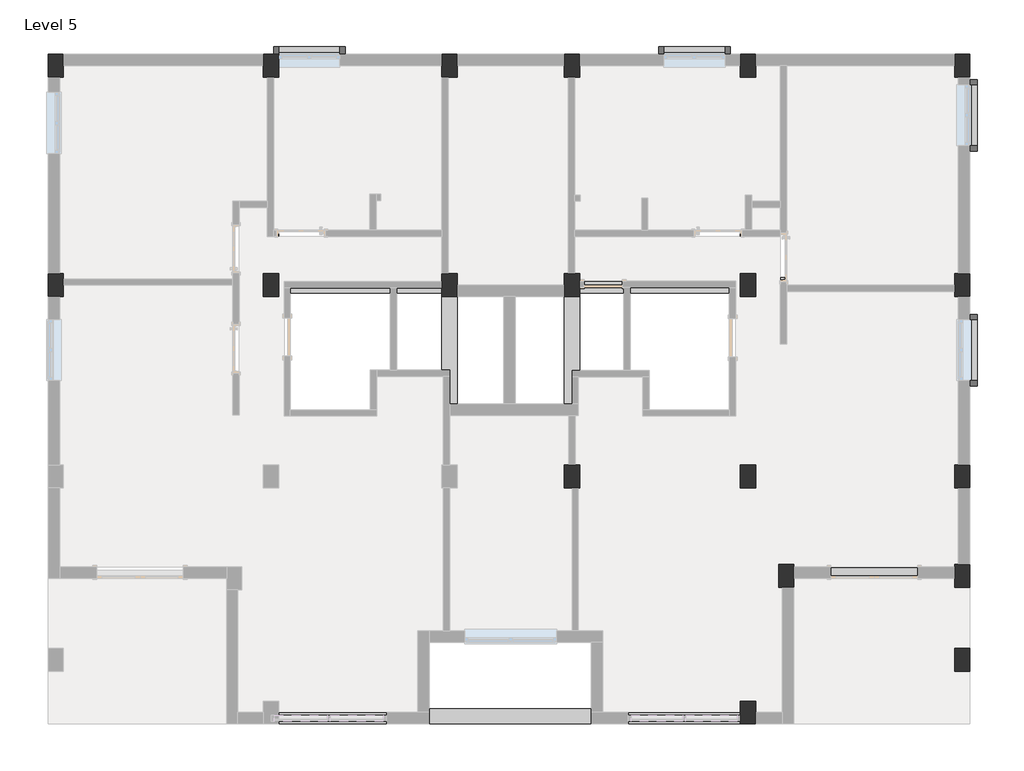
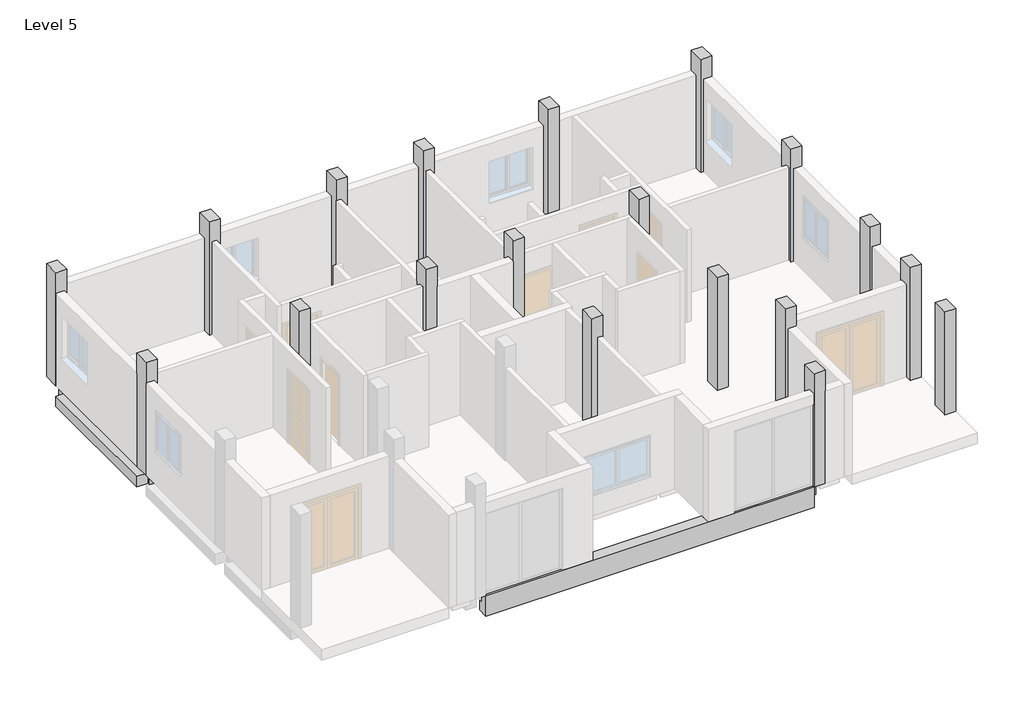
# One storey, part 3 of 3: 30 beams, 19 columns, 4 proxies.
"""IFC4 building model written with IfcOpenShell, lengths in millimetres."""

from ifc_helpers import new_model, si_unit, frame, origin, place, context, project, spatial, polyline, outline, extrude, faceted_brep, transform, mapped, element, save
from components import generic_models_10_generic_models_5_40bb8100, generic_models_13_generic_models_13_6edbfaa0, column_61ecc76d

model = new_model("IFC4")

# Units and contexts
model_context = context("Model", 3, world=origin())
ifc_project = project(units=[si_unit("LENGTHUNIT", "METRE", prefix="MILLI")], contexts=[model_context])

# Site, building, storey
site = spatial("IfcSite", under=ifc_project)
building = spatial("IfcBuilding", under=site)
storey = spatial("IfcBuildingStorey", under=building, Name="Level 5", Elevation=6400.8)

# Beams
placement = place(None, origin())
element("IfcBeam", 1, ObjectType="Concrete-Rectangular Beam : 12 x 24", at=placement, inside=storey, context=model_context, shape_type="SweptSolid", body=[
    extrude(outline(polyline([(-8839.9786397, -1604.6061634), (-8839.9786397, -1299.8061634), (-4852.9175798, -1299.8061634), (-4852.9175798, -1604.6061634), (-8839.9786397, -1604.6061634)])), frame((0.0, 0.0, 5791.2), z_axis=(0.0, 0.0, 1.0), x_axis=(1.0, 0.0, 0.0)), (0.0, 0.0, 1.0), 304.8),
])
element("IfcBeam", 2, ObjectType="Concrete-Rectangular Beam : 12 x 24", at=placement, inside=storey, context=model_context, shape_type="SweptSolid", body=[
    extrude(outline(polyline([(-1296.9175798, -1604.6061634), (-4548.1175798, -1604.6061634), (-4548.1175798, -1299.8061634), (-1296.9175798, -1299.8061634), (-1296.9175798, -1604.6061634)])), frame((0.0, 0.0, 5791.2), z_axis=(0.0, 0.0, 1.0), x_axis=(1.0, 0.0, 0.0)), (0.0, 0.0, 1.0), 304.8),
])
element("IfcBeam", 3, ObjectType="Concrete-Rectangular Beam : 12 x 24", at=placement, inside=storey, context=model_context, shape_type="SweptSolid", body=[
    extrude(outline(polyline([(1141.4824202, -1604.6061634), (-992.1175798, -1604.6061634), (-992.1175798, -1299.8061634), (1141.4824202, -1299.8061634), (1141.4824202, -1604.6061634)])), frame((0.0, 0.0, 5791.2), z_axis=(0.0, 0.0, 1.0), x_axis=(1.0, 0.0, 0.0)), (0.0, 0.0, 1.0), 304.8),
])
element("IfcBeam", 4, ObjectType="Concrete-Rectangular Beam : 12 x 24", at=placement, inside=storey, context=model_context, shape_type="SweptSolid", body=[
    extrude(outline(polyline([(4646.6824202, -1604.6061634), (1446.2824202, -1604.6061634), (1446.2824202, -1299.8061634), (4646.6824202, -1299.8061634), (4646.6824202, -1604.6061634)])), frame((0.0, 0.0, 5791.2), z_axis=(0.0, 0.0, 1.0), x_axis=(1.0, 0.0, 0.0)), (0.0, 0.0, 1.0), 304.8),
])
element("IfcBeam", 5, ObjectType="Concrete-Rectangular Beam : 12 x 24", at=placement, inside=storey, context=model_context, shape_type="SweptSolid", body=[
    extrude(outline(polyline([(8913.9345022, -1604.6061634), (4951.5345022, -1604.6061634), (4951.5345022, -1299.8061634), (8913.9345022, -1299.8061634), (8913.9345022, -1604.6061634)])), frame((0.0, 0.0, 5791.2), z_axis=(0.0, 0.0, 1.0), x_axis=(1.0, 0.0, 0.0)), (0.0, 0.0, 1.0), 304.8),
])
element("IfcBeam", 6, ObjectType="Concrete-Rectangular Beam : 12 x 24", at=placement, inside=storey, context=model_context, shape_type="SweptSolid", body=[
    extrude(outline(polyline([(8913.8824202, -5600.6620333), (8913.8824202, -1680.8061634), (9218.6824202, -1680.8061634), (9218.6824202, -5600.6620333), (8913.8824202, -5600.6620333)])), frame((0.0, 0.0, 5791.2), z_axis=(0.0, 0.0, 1.0), x_axis=(1.0, 0.0, 0.0)), (0.0, 0.0, 1.0), 304.8),
])
element("IfcBeam", 7, ObjectType="Concrete-Rectangular Beam : 12 x 24", at=placement, inside=storey, context=model_context, shape_type="SweptSolid", body=[
    extrude(outline(polyline([(8913.8824202, -9410.6620333), (8913.8824202, -6057.8620333), (9218.6824202, -6057.8620333), (9218.6824202, -9410.6620333), (8913.8824202, -9410.6620333)])), frame((0.0, 0.0, 5791.2), z_axis=(0.0, 0.0, 1.0), x_axis=(1.0, 0.0, 0.0)), (0.0, 0.0, 1.0), 304.8),
])
element("IfcBeam", 8, ObjectType="Concrete-Rectangular Beam : 12 x 24", at=placement, inside=storey, context=model_context, shape_type="SweptSolid", body=[
    extrude(outline(polyline([(8913.8824202, -11391.8620333), (8913.8824202, -9867.8620333), (9218.6824202, -9867.8620333), (9218.6824202, -11391.8620333), (8913.8824202, -11391.8620333)])), frame((0.0, 0.0, 5791.2), z_axis=(0.0, 0.0, 1.0), x_axis=(1.0, 0.0, 0.0)), (0.0, 0.0, 1.0), 304.8),
])
element("IfcBeam", 9, ObjectType="Concrete-Rectangular Beam : 12 x 24", at=placement, inside=storey, context=model_context, shape_type="SweptSolid", body=[
    extrude(outline(polyline([(-9144.7786397, -5600.6620333), (-9144.7786397, -1680.8061634), (-8839.9786397, -1680.8061634), (-8839.9786397, -5600.6620333), (-9144.7786397, -5600.6620333)])), frame((0.0, 0.0, 5791.2), z_axis=(0.0, 0.0, 1.0), x_axis=(1.0, 0.0, 0.0)), (0.0, 0.0, 1.0), 304.8),
])
element("IfcBeam", 10, ObjectType="Concrete-Rectangular Beam : 12 x 24", at=placement, inside=storey, context=model_context, shape_type="SweptSolid", body=[
    extrude(outline(polyline([(4951.4824202, -5676.8620333), (8913.8824202, -5676.8620333), (8913.8824202, -5981.6620333), (4951.4824202, -5981.6620333), (4951.4824202, -5676.8620333)])), frame((0.0, 0.0, 5791.2), z_axis=(0.0, 0.0, 1.0), x_axis=(1.0, 0.0, 0.0)), (0.0, 0.0, 1.0), 304.8),
])
element("IfcBeam", 11, ObjectType="Concrete-Rectangular Beam : 12 x 24", at=placement, inside=storey, context=model_context, shape_type="SweptSolid", body=[
    extrude(outline(polyline([(1446.2824202, -5676.8620333), (4646.6824202, -5676.8620333), (4646.6824202, -5981.6620333), (1446.2824202, -5981.6620333), (1446.2824202, -5676.8620333)])), frame((0.0, 0.0, 5791.2), z_axis=(0.0, 0.0, 1.0), x_axis=(1.0, 0.0, 0.0)), (0.0, 0.0, 1.0), 304.8),
])
element("IfcBeam", 12, ObjectType="Concrete-Rectangular Beam : 12 x 24", at=placement, inside=storey, context=model_context, shape_type="SweptSolid", body=[
    extrude(outline(polyline([(-992.1175798, -5676.8620333), (1141.4824202, -5676.8620333), (1141.4824202, -5981.6620333), (-992.1175798, -5981.6620333), (-992.1175798, -5676.8620333)])), frame((0.0, 0.0, 5791.2), z_axis=(0.0, 0.0, 1.0), x_axis=(1.0, 0.0, 0.0)), (0.0, 0.0, 1.0), 304.8),
])
element("IfcBeam", 13, ObjectType="Concrete-Rectangular Beam : 12 x 24", at=placement, inside=storey, context=model_context, shape_type="SweptSolid", body=[
    extrude(outline(polyline([(-4548.1175798, -5676.8620333), (-1296.9175798, -5676.8620333), (-1296.9175798, -5981.6620333), (-4548.1175798, -5981.6620333), (-4548.1175798, -5676.8620333)])), frame((0.0, 0.0, 5791.2), z_axis=(0.0, 0.0, 1.0), x_axis=(1.0, 0.0, 0.0)), (0.0, 0.0, 1.0), 304.8),
])
element("IfcBeam", 14, ObjectType="Concrete-Rectangular Beam : 12 x 24", at=placement, inside=storey, context=model_context, shape_type="SweptSolid", body=[
    extrude(outline(polyline([(-8839.9786397, -5676.8620333), (-4852.9175798, -5676.8620333), (-4852.9175798, -5981.6620333), (-8839.9786397, -5981.6620333), (-8839.9786397, -5676.8620333)])), frame((0.0, 0.0, 5791.2), z_axis=(0.0, 0.0, 1.0), x_axis=(1.0, 0.0, 0.0)), (0.0, 0.0, 1.0), 304.8),
])
element("IfcBeam", 15, ObjectType="Concrete-Rectangular Beam : 12 x 24", at=placement, inside=storey, context=model_context, shape_type="SweptSolid", body=[
    extrude(outline(polyline([(1446.2824202, -9791.6620333), (1446.2824202, -9486.8620333), (4646.6824202, -9486.8620333), (4646.6824202, -9791.6620333), (1446.2824202, -9791.6620333)])), frame((0.0, 0.0, 5791.2), z_axis=(0.0, 0.0, 1.0), x_axis=(1.0, 0.0, 0.0)), (0.0, 0.0, 1.0), 304.8),
])
element("IfcBeam", 16, ObjectType="Concrete-Rectangular Beam : 12 x 24", at=placement, inside=storey, context=model_context, shape_type="Brep", body=[
    faceted_brep([(4646.6824202, -9867.8620333, 5791.2), (4646.6824202, -11772.8620333, 5791.2), (4646.6824202, -11772.8620333, 6096.0), (4646.6824202, -9867.8620333, 6096.0), (4951.4824202, -9867.8620333, 5791.2), (4951.4824202, -11468.0620333, 5791.2), (4951.4824202, -11772.8620333, 5791.2), (4951.4824202, -9867.8620333, 6096.0), (4951.4824202, -11468.0620333, 6096.0), (4951.4824202, -11772.8620333, 6096.0)], [[[0, 1, 2, 3]], [[0, 4, 5, 6, 1]], [[6, 5, 4, 7, 8, 9]], [[4, 0, 3, 7]], [[3, 2, 9, 8, 7]], [[1, 6, 9, 2]]]),
])
element("IfcBeam", 17, ObjectType="Concrete-Rectangular Beam : 12 x 24", at=placement, inside=storey, context=model_context, shape_type="SweptSolid", body=[
    extrude(outline(polyline([(4951.4824202, -11772.8620333), (4951.4824202, -11468.0620333), (5408.6824202, -11468.0620333), (5408.6824202, -11772.8620333), (4951.4824202, -11772.8620333)])), frame((0.0, 0.0, 5791.2), z_axis=(0.0, 0.0, 1.0), x_axis=(1.0, 0.0, 0.0)), (0.0, 0.0, 1.0), 304.8),
])
element("IfcBeam", 18, ObjectType="Concrete-Rectangular Beam : 12 x 24", at=placement, inside=storey, context=model_context, shape_type="SweptSolid", body=[
    extrude(outline(polyline([(8913.8824202, -11772.8620333), (5713.4824202, -11772.8620333), (5713.4824202, -11468.0620333), (8913.8824202, -11468.0620333), (8913.8824202, -11772.8620333)])), frame((0.0, 0.0, 5791.2), z_axis=(0.0, 0.0, 1.0), x_axis=(1.0, 0.0, 0.0)), (0.0, 0.0, 1.0), 304.8),
])
element("IfcBeam", 19, ObjectType="Concrete-Rectangular Beam : 12 x 24", at=placement, inside=storey, context=model_context, shape_type="SweptSolid", body=[
    extrude(outline(polyline([(4646.6824202, -14272.0402089), (4646.6824202, -14576.8402089), (-4548.1175798, -14576.8402089), (-4548.1175798, -14272.0402089), (4646.6824202, -14272.0402089)])), frame((0.0, 0.0, 5791.2), z_axis=(0.0, 0.0, 1.0), x_axis=(1.0, 0.0, 0.0)), (0.0, 0.0, 1.0), 609.6),
])
element("IfcBeam", 20, ObjectType="Concrete-Rectangular Beam : 12 x 24", at=placement, inside=storey, context=model_context, shape_type="SweptSolid", body=[
    extrude(outline(polyline([(4951.4824202, -14119.6402089), (4646.6824202, -14119.6402089), (4646.6824202, -11772.8620333), (4951.4824202, -11772.8620333), (4951.4824202, -14119.6402089)])), frame((0.0, 0.0, 5791.2), z_axis=(0.0, 0.0, 1.0), x_axis=(1.0, 0.0, 0.0)), (0.0, 0.0, 1.0), 304.8),
])
element("IfcBeam", 21, ObjectType="Concrete-Rectangular Beam : 12 x 24", at=placement, inside=storey, context=model_context, shape_type="SweptSolid", body=[
    extrude(outline(polyline([(-4852.9175798, -5600.6620333), (-4852.9175798, -1680.8061634), (-4548.1175798, -1680.8061634), (-4548.1175798, -5600.6620333), (-4852.9175798, -5600.6620333)])), frame((0.0, 0.0, 5791.2), z_axis=(0.0, 0.0, 1.0), x_axis=(1.0, 0.0, 0.0)), (0.0, 0.0, 1.0), 304.8),
])
element("IfcBeam", 22, ObjectType="Concrete-Rectangular Beam : 12 x 24", at=placement, inside=storey, context=model_context, shape_type="SweptSolid", body=[
    extrude(outline(polyline([(-4852.9175798, -9410.6620333), (-4852.9175798, -6057.8620333), (-4548.1175798, -6057.8620333), (-4548.1175798, -9410.6620333), (-4852.9175798, -9410.6620333)])), frame((0.0, 0.0, 5791.2), z_axis=(0.0, 0.0, 1.0), x_axis=(1.0, 0.0, 0.0)), (0.0, 0.0, 1.0), 304.8),
])
element("IfcBeam", 23, ObjectType="Concrete-Rectangular Beam : 12 x 24", at=placement, inside=storey, context=model_context, shape_type="SweptSolid", body=[
    extrude(outline(polyline([(-1296.9175798, -5600.6620333), (-1296.9175798, -1680.8061634), (-992.1175798, -1680.8061634), (-992.1175798, -5600.6620333), (-1296.9175798, -5600.6620333)])), frame((0.0, 0.0, 5791.2), z_axis=(0.0, 0.0, 1.0), x_axis=(1.0, 0.0, 0.0)), (0.0, 0.0, 1.0), 304.8),
])
element("IfcBeam", 24, ObjectType="Concrete-Rectangular Beam : 12 x 24", at=placement, inside=storey, context=model_context, shape_type="SweptSolid", body=[
    extrude(outline(polyline([(-1296.9175798, -9410.6620333), (-1296.9175798, -6057.8620333), (-992.1175798, -6057.8620333), (-992.1175798, -9410.6620333), (-1296.9175798, -9410.6620333)])), frame((0.0, 0.0, 5791.2), z_axis=(0.0, 0.0, 1.0), x_axis=(1.0, 0.0, 0.0)), (0.0, 0.0, 1.0), 304.8),
])
element("IfcBeam", 25, ObjectType="Concrete-Rectangular Beam : 12 x 24", at=placement, inside=storey, context=model_context, shape_type="SweptSolid", body=[
    extrude(outline(polyline([(1446.2824202, -6057.8620333), (1446.2824202, -9410.6620333), (1141.4824202, -9410.6620333), (1141.4824202, -6057.8620333), (1446.2824202, -6057.8620333)])), frame((0.0, 0.0, 5791.2), z_axis=(0.0, 0.0, 1.0), x_axis=(1.0, 0.0, 0.0)), (0.0, 0.0, 1.0), 304.8),
])
element("IfcBeam", 26, ObjectType="Concrete-Rectangular Beam : 12 x 24", at=placement, inside=storey, context=model_context, shape_type="SweptSolid", body=[
    extrude(outline(polyline([(1446.2824202, -1680.8061634), (1446.2824202, -5600.6620333), (1141.4824202, -5600.6620333), (1141.4824202, -1680.8061634), (1446.2824202, -1680.8061634)])), frame((0.0, 0.0, 5791.2), z_axis=(0.0, 0.0, 1.0), x_axis=(1.0, 0.0, 0.0)), (0.0, 0.0, 1.0), 304.8),
])
element("IfcBeam", 27, ObjectType="Concrete-Rectangular Beam : 12 x 24", at=placement, inside=storey, context=model_context, shape_type="SweptSolid", body=[
    extrude(outline(polyline([(4646.6824202, -5600.6620333), (4646.6824202, -1680.8061634), (4951.4824202, -1680.8061634), (4951.4824202, -5600.6620333), (4646.6824202, -5600.6620333)])), frame((0.0, 0.0, 5791.2), z_axis=(0.0, 0.0, 1.0), x_axis=(1.0, 0.0, 0.0)), (0.0, 0.0, 1.0), 304.8),
])
element("IfcBeam", 28, ObjectType="Concrete-Rectangular Beam : 12 x 24", at=placement, inside=storey, context=model_context, shape_type="SweptSolid", body=[
    extrude(outline(polyline([(4646.6824202, -9410.6620333), (4646.6824202, -6057.8620333), (4951.4824202, -6057.8620333), (4951.4824202, -9410.6620333), (4646.6824202, -9410.6620333)])), frame((0.0, 0.0, 5791.2), z_axis=(0.0, 0.0, 1.0), x_axis=(1.0, 0.0, 0.0)), (0.0, 0.0, 1.0), 304.8),
])
element("IfcBeam", 29, ObjectType="Concrete-Rectangular Beam : 12 x 24", at=placement, inside=storey, context=model_context, shape_type="SweptSolid", body=[
    extrude(outline(polyline([(4951.4824202, -9486.8620333), (8913.8824202, -9486.8620333), (8913.8824202, -9791.6620333), (4951.4824202, -9791.6620333), (4951.4824202, -9486.8620333)])), frame((0.0, 0.0, 5791.2), z_axis=(0.0, 0.0, 1.0), x_axis=(1.0, 0.0, 0.0)), (0.0, 0.0, 1.0), 304.8),
])
element("IfcBeam", 30, ObjectType="Concrete-Rectangular Beam : 12 x 24", at=placement, inside=storey, context=model_context, shape_type="SweptSolid", body=[
    extrude(outline(polyline([(1141.4824202, -9486.8620333), (1141.4824202, -9791.6620333), (-992.1175798, -9791.6620333), (-992.1175798, -9486.8620333), (1141.4824202, -9486.8620333)])), frame((0.0, 0.0, 5791.2), z_axis=(0.0, 0.0, 1.0), x_axis=(1.0, 0.0, 0.0)), (0.0, 0.0, 1.0), 609.6),
])

# Proxies
generic_models_10_generic_models_5_shape = generic_models_10_generic_models_5_40bb8100(model_context)
element("IfcBuildingElementProxy", 31, Name="Generic Models 12 : Generic Models 5", ObjectType="Generic Models 12 : Generic Models 5", at=placement, inside=storey, context=model_context, shape_type="MappedRepresentation", body=[
    mapped(generic_models_10_generic_models_5_shape, transform((0.0, 0.0, -3048.0), x_axis=(1.0, 0.0, 0.0), y_axis=(0.0, 1.0, 0.0), z_axis=(0.0, 0.0, 1.0))),
])
generic_models_13_generic_models_13_shape = generic_models_13_generic_models_13_6edbfaa0(model_context)
element("IfcBuildingElementProxy", 32, Name="Generic Models 15 : Generic Models 13", ObjectType="Generic Models 15 : Generic Models 13", at=placement, inside=storey, context=model_context, shape_type="MappedRepresentation", body=[
    mapped(generic_models_13_generic_models_13_shape, transform((0.0, 0.0, -3048.0), x_axis=(1.0, 0.0, 0.0), y_axis=(0.0, 1.0, 0.0), z_axis=(0.0, 0.0, 1.0))),
])
element("IfcBuildingElementProxy", 33, Name="Generic Models 18 : Generic Models 13", ObjectType="Generic Models 18 : Generic Models 13", at=placement, inside=storey, context=model_context, shape_type="MappedRepresentation", body=[
    mapped(generic_models_13_generic_models_13_shape, transform((-7670.8, 0.0, -3048.0), x_axis=(1.0, 0.0, 0.0), y_axis=(0.0, 1.0, 0.0), z_axis=(0.0, 0.0, 1.0))),
])
element("IfcBuildingElementProxy", 34, Name="Generic Models 7 : Generic Models 5", ObjectType="Generic Models 7 : Generic Models 5", at=placement, inside=storey, context=model_context, shape_type="MappedRepresentation", body=[
    mapped(generic_models_10_generic_models_5_shape, transform((0.0, 4681.8558699, -3048.0), x_axis=(1.0, 0.0, 0.0), y_axis=(0.0, 1.0, 0.0), z_axis=(0.0, 0.0, 1.0))),
])

# Columns
element("IfcColumn", 35, ObjectType="Concrete-Rectangular-Column : 1'6\" X 1' COLUMN", at=placement, inside=storey, context=model_context, shape_type="Brep", body=[
    faceted_brep([(-8839.9786397, -1223.6061634, 6400.8), (-8839.9786397, -1680.8061634, 6400.8), (-9144.7786397, -1680.8061634, 6400.8), (-9144.7786397, -1223.6061634, 6400.8), (-8839.9786397, -1223.6061634, 9753.6), (-8839.9786397, -1299.8061634, 9753.6), (-8839.9786397, -1604.6061634, 9753.6), (-8839.9786397, -1680.8061634, 9753.6), (-8839.9786397, -1680.8061634, 9144.0), (-8839.9786397, -1680.8061634, 8839.2), (-8839.9786397, -1680.8061634, 6705.6), (-9144.7786397, -1680.8061634, 9753.6), (-9144.7786397, -1680.8061634, 9144.0), (-9144.7786397, -1680.8061634, 8839.2), (-9144.7786397, -1680.8061634, 6705.6), (-9144.7786397, -1223.6061634, 9753.6)], [[[0, 1, 2, 3]], [[4, 5, 6, 7, 8, 9, 10, 1, 0]], [[7, 11, 12, 13, 14, 2, 1, 10, 9, 8]], [[11, 15, 3, 2, 14, 13, 12]], [[15, 4, 0, 3]], [[4, 15, 11, 7, 6, 5]]]),
])
element("IfcColumn", 36, ObjectType="Concrete-Rectangular-Column : 1'6\" X 1' COLUMN", at=placement, inside=storey, context=model_context, shape_type="Brep", body=[
    faceted_brep([(-4548.1175798, -1223.6061634, 6400.8), (-4548.1175798, -1680.8061634, 6400.8), (-4852.9175798, -1680.8061634, 6400.8), (-4852.9175798, -1223.6061634, 6400.8), (-4548.1175798, -1223.6061634, 9753.6), (-4548.1175798, -1299.8061634, 9753.6), (-4548.1175798, -1604.6061634, 9753.6), (-4548.1175798, -1680.8061634, 9753.6), (-4548.1175798, -1680.8061634, 9144.0), (-4548.1175798, -1680.8061634, 8839.2), (-4548.1175798, -1680.8061634, 6705.6), (-4852.9175798, -1680.8061634, 9753.6), (-4852.9175798, -1680.8061634, 9144.0), (-4852.9175798, -1680.8061634, 8839.2), (-4852.9175798, -1680.8061634, 6705.6), (-4852.9175798, -1223.6061634, 9753.6)], [[[0, 1, 2, 3]], [[4, 5, 6, 7, 8, 9, 10, 1, 0]], [[7, 11, 12, 13, 14, 2, 1, 10, 9, 8]], [[11, 15, 3, 2, 14, 13, 12]], [[15, 4, 0, 3]], [[4, 15, 11, 7, 6, 5]]]),
])
element("IfcColumn", 37, ObjectType="Concrete-Rectangular-Column : 1'6\" X 1' COLUMN", at=placement, inside=storey, context=model_context, shape_type="Brep", body=[
    faceted_brep([(-992.1175798, -1223.6061634, 6400.8), (-992.1175798, -1680.8061634, 6400.8), (-1296.9175798, -1680.8061634, 6400.8), (-1296.9175798, -1223.6061634, 6400.8), (-992.1175798, -1223.6061634, 9753.6), (-992.1175798, -1299.8061634, 9753.6), (-992.1175798, -1604.6061634, 9753.6), (-992.1175798, -1680.8061634, 9753.6), (-992.1175798, -1680.8061634, 9144.0), (-992.1175798, -1680.8061634, 8839.2), (-992.1175798, -1680.8061634, 6705.6), (-1296.9175798, -1680.8061634, 9753.6), (-1296.9175798, -1680.8061634, 9144.0), (-1296.9175798, -1680.8061634, 8839.2), (-1296.9175798, -1680.8061634, 6705.6), (-1296.9175798, -1604.6061634, 9753.6), (-1296.9175798, -1299.8061634, 9753.6), (-1296.9175798, -1223.6061634, 9753.6)], [[[0, 1, 2, 3]], [[4, 5, 6, 7, 8, 9, 10, 1, 0]], [[7, 11, 12, 13, 14, 2, 1, 10, 9, 8]], [[11, 15, 16, 17, 3, 2, 14, 13, 12]], [[17, 4, 0, 3]], [[4, 17, 16, 15, 11, 7, 6, 5]]]),
])
element("IfcColumn", 38, ObjectType="Concrete-Rectangular-Column : 1'6\" X 1' COLUMN", at=placement, inside=storey, context=model_context, shape_type="Brep", body=[
    faceted_brep([(1446.2824202, -1223.6061634, 6400.8), (1446.2824202, -1680.8061634, 6400.8), (1141.4824202, -1680.8061634, 6400.8), (1141.4824202, -1223.6061634, 6400.8), (1446.2824202, -1223.6061634, 9753.6), (1446.2824202, -1299.8061634, 9753.6), (1446.2824202, -1604.6061634, 9753.6), (1446.2824202, -1680.8061634, 9753.6), (1446.2824202, -1680.8061634, 9144.0), (1446.2824202, -1680.8061634, 8839.2), (1446.2824202, -1680.8061634, 6705.6), (1141.4824202, -1680.8061634, 9753.6), (1141.4824202, -1680.8061634, 9144.0), (1141.4824202, -1680.8061634, 8839.2), (1141.4824202, -1680.8061634, 6705.6), (1141.4824202, -1604.6061634, 9753.6), (1141.4824202, -1299.8061634, 9753.6), (1141.4824202, -1223.6061634, 9753.6)], [[[0, 1, 2, 3]], [[4, 5, 6, 7, 8, 9, 10, 1, 0]], [[7, 11, 12, 13, 14, 2, 1, 10, 9, 8]], [[11, 15, 16, 17, 3, 2, 14, 13, 12]], [[17, 4, 0, 3]], [[4, 17, 16, 15, 11, 7, 6, 5]]]),
])
element("IfcColumn", 39, ObjectType="Concrete-Rectangular-Column : 1'6\" X 1' COLUMN", at=placement, inside=storey, context=model_context, shape_type="Brep", body=[
    faceted_brep([(4951.4824202, -1223.6061634, 6400.8), (4951.4824202, -1680.8061634, 6400.8), (4646.6824202, -1680.8061634, 6400.8), (4646.6824202, -1223.6061634, 6400.8), (4951.4824202, -1223.6061634, 9753.6), (4951.4824202, -1680.8061634, 9753.6), (4951.4824202, -1680.8061634, 9144.0), (4951.4824202, -1680.8061634, 8839.2), (4951.4824202, -1680.8061634, 6705.6), (4646.6824202, -1680.8061634, 9753.6), (4646.6824202, -1680.8061634, 9144.0), (4646.6824202, -1680.8061634, 8839.2), (4646.6824202, -1680.8061634, 6705.6), (4646.6824202, -1604.6061634, 9753.6), (4646.6824202, -1299.8061634, 9753.6), (4646.6824202, -1223.6061634, 9753.6)], [[[0, 1, 2, 3]], [[4, 5, 6, 7, 8, 1, 0]], [[5, 9, 10, 11, 12, 2, 1, 8, 7, 6]], [[9, 13, 14, 15, 3, 2, 12, 11, 10]], [[15, 4, 0, 3]], [[4, 15, 14, 13, 9, 5]]]),
])
element("IfcColumn", 40, ObjectType="Concrete-Rectangular-Column : 1'6\" X 1' COLUMN", at=placement, inside=storey, context=model_context, shape_type="Brep", body=[
    faceted_brep([(9218.6824202, -1223.6061634, 6400.8), (9218.6824202, -1680.8061634, 6400.8), (8913.8824202, -1680.8061634, 6400.8), (8913.8824202, -1223.6061634, 6400.8), (9218.6824202, -1223.6061634, 9753.6), (9218.6824202, -1680.8061634, 9753.6), (9218.6824202, -1680.8061634, 9144.0), (9218.6824202, -1680.8061634, 8839.2), (9218.6824202, -1680.8061634, 6705.6), (8913.8824202, -1680.8061634, 9753.6), (8913.8824202, -1680.8061634, 9144.0), (8913.8824202, -1680.8061634, 8839.2), (8913.8824202, -1680.8061634, 6705.6), (8913.8824202, -1223.6061634, 9753.6)], [[[0, 1, 2, 3]], [[4, 5, 6, 7, 8, 1, 0]], [[5, 9, 10, 11, 12, 2, 1, 8, 7, 6]], [[9, 13, 3, 2, 12, 11, 10]], [[13, 4, 0, 3]], [[4, 13, 9, 5]]]),
])
element("IfcColumn", 41, ObjectType="Concrete-Rectangular-Column : 1'6\" X 1' COLUMN", at=placement, inside=storey, context=model_context, shape_type="Brep", body=[
    faceted_brep([(9218.6824202, -5600.6620333, 6400.8), (9218.6824202, -6057.8620333, 6400.8), (8913.8824202, -6057.8620333, 6400.8), (8913.8824202, -5600.6620333, 6400.8), (9218.6824202, -5600.6620333, 9753.6), (9218.6824202, -6057.8620333, 9753.6), (9218.6824202, -6057.8620333, 9144.0), (9218.6824202, -6057.8620333, 8839.2), (9218.6824202, -6057.8620333, 6705.6), (9218.6824202, -5600.6620333, 6705.6), (9218.6824202, -5600.6620333, 8839.2), (9218.6824202, -5600.6620333, 9144.0), (8913.8824202, -6057.8620333, 9753.6), (8913.8824202, -6057.8620333, 9144.0), (8913.8824202, -6057.8620333, 8839.2), (8913.8824202, -6057.8620333, 6705.6), (8913.8824202, -5981.6620333, 9753.6), (8913.8824202, -5676.8620333, 9753.6), (8913.8824202, -5600.6620333, 9753.6), (8913.8824202, -5600.6620333, 9144.0), (8913.8824202, -5600.6620333, 8839.2), (8913.8824202, -5600.6620333, 6705.6)], [[[0, 1, 2, 3]], [[4, 5, 6, 7, 8, 1, 0, 9, 10, 11]], [[5, 12, 13, 14, 15, 2, 1, 8, 7, 6]], [[12, 16, 17, 18, 19, 20, 21, 3, 2, 15, 14, 13]], [[18, 4, 11, 10, 9, 0, 3, 21, 20, 19]], [[4, 18, 17, 16, 12, 5]]]),
])
element("IfcColumn", 42, ObjectType="Concrete-Rectangular-Column : 1'6\" X 1' COLUMN", at=placement, inside=storey, context=model_context, shape_type="Brep", body=[
    faceted_brep([(4951.4824202, -5600.6620333, 6400.8), (4951.4824202, -6057.8620333, 6400.8), (4646.6824202, -6057.8620333, 6400.8), (4646.6824202, -5600.6620333, 6400.8), (4951.4824202, -5600.6620333, 9753.6), (4951.4824202, -5676.8620333, 9753.6), (4951.4824202, -5981.6620333, 9753.6), (4951.4824202, -6057.8620333, 9753.6), (4951.4824202, -6057.8620333, 9144.0), (4951.4824202, -6057.8620333, 8839.2), (4951.4824202, -6057.8620333, 6705.6), (4951.4824202, -5600.6620333, 6705.6), (4951.4824202, -5600.6620333, 8839.2), (4951.4824202, -5600.6620333, 9144.0), (4646.6824202, -6057.8620333, 9753.6), (4646.6824202, -6057.8620333, 9144.0), (4646.6824202, -6057.8620333, 8839.2), (4646.6824202, -6057.8620333, 6705.6), (4646.6824202, -5981.6620333, 9753.6), (4646.6824202, -5676.8620333, 9753.6), (4646.6824202, -5600.6620333, 9753.6), (4646.6824202, -5600.6620333, 9144.0), (4646.6824202, -5600.6620333, 8839.2), (4646.6824202, -5600.6620333, 6705.6)], [[[0, 1, 2, 3]], [[4, 5, 6, 7, 8, 9, 10, 1, 0, 11, 12, 13]], [[7, 14, 15, 16, 17, 2, 1, 10, 9, 8]], [[14, 18, 19, 20, 21, 22, 23, 3, 2, 17, 16, 15]], [[20, 4, 13, 12, 11, 0, 3, 23, 22, 21]], [[4, 20, 19, 18, 14, 7, 6, 5]]]),
])
element("IfcColumn", 43, ObjectType="Concrete-Rectangular-Column : 1'6\" X 1' COLUMN", at=placement, inside=storey, context=model_context, shape_type="Brep", body=[
    faceted_brep([(1446.2824202, -5600.6620333, 6400.8), (1446.2824202, -6057.8620333, 6400.8), (1141.4824202, -6057.8620333, 6400.8), (1141.4824202, -5600.6620333, 6400.8), (1446.2824202, -5600.6620333, 9753.6), (1446.2824202, -5676.8620333, 9753.6), (1446.2824202, -5981.6620333, 9753.6), (1446.2824202, -6057.8620333, 9753.6), (1446.2824202, -6057.8620333, 9144.0), (1446.2824202, -6057.8620333, 8839.2), (1446.2824202, -6057.8620333, 6705.6), (1446.2824202, -5600.6620333, 6705.6), (1446.2824202, -5600.6620333, 8839.2), (1446.2824202, -5600.6620333, 9144.0), (1141.4824202, -6057.8620333, 9753.6), (1141.4824202, -6057.8620333, 9144.0), (1141.4824202, -6057.8620333, 8839.2), (1141.4824202, -6057.8620333, 6705.6), (1141.4824202, -5981.6620333, 9753.6), (1141.4824202, -5676.8620333, 9753.6), (1141.4824202, -5600.6620333, 9753.6), (1141.4824202, -5600.6620333, 9144.0), (1141.4824202, -5600.6620333, 8839.2), (1141.4824202, -5600.6620333, 6705.6)], [[[0, 1, 2, 3]], [[4, 5, 6, 7, 8, 9, 10, 1, 0, 11, 12, 13]], [[7, 14, 15, 16, 17, 2, 1, 10, 9, 8]], [[14, 18, 19, 20, 21, 22, 23, 3, 2, 17, 16, 15]], [[20, 4, 13, 12, 11, 0, 3, 23, 22, 21]], [[4, 20, 19, 18, 14, 7, 6, 5]]]),
])
element("IfcColumn", 44, ObjectType="Concrete-Rectangular-Column : 1'6\" X 1' COLUMN", at=placement, inside=storey, context=model_context, shape_type="Brep", body=[
    faceted_brep([(-992.1175798, -5600.6620333, 6400.8), (-992.1175798, -6057.8620333, 6400.8), (-1296.9175798, -6057.8620333, 6400.8), (-1296.9175798, -5600.6620333, 6400.8), (-992.1175798, -5600.6620333, 9753.6), (-992.1175798, -5676.8620333, 9753.6), (-992.1175798, -5981.6620333, 9753.6), (-992.1175798, -6057.8620333, 9753.6), (-992.1175798, -6057.8620333, 9144.0), (-992.1175798, -6057.8620333, 8839.2), (-992.1175798, -6057.8620333, 6705.6), (-992.1175798, -5600.6620333, 6705.6), (-992.1175798, -5600.6620333, 8839.2), (-992.1175798, -5600.6620333, 9144.0), (-1296.9175798, -6057.8620333, 9753.6), (-1296.9175798, -6057.8620333, 9144.0), (-1296.9175798, -6057.8620333, 8839.2), (-1296.9175798, -6057.8620333, 6705.6), (-1296.9175798, -5981.6620333, 9753.6), (-1296.9175798, -5676.8620333, 9753.6), (-1296.9175798, -5600.6620333, 9753.6), (-1296.9175798, -5600.6620333, 9144.0), (-1296.9175798, -5600.6620333, 8839.2), (-1296.9175798, -5600.6620333, 6705.6)], [[[0, 1, 2, 3]], [[4, 5, 6, 7, 8, 9, 10, 1, 0, 11, 12, 13]], [[7, 14, 15, 16, 17, 2, 1, 10, 9, 8]], [[14, 18, 19, 20, 21, 22, 23, 3, 2, 17, 16, 15]], [[20, 4, 13, 12, 11, 0, 3, 23, 22, 21]], [[4, 20, 19, 18, 14, 7, 6, 5]]]),
])
element("IfcColumn", 45, ObjectType="Concrete-Rectangular-Column : 1'6\" X 1' COLUMN", at=placement, inside=storey, context=model_context, shape_type="Brep", body=[
    faceted_brep([(-4548.1175798, -5600.6620333, 6400.8), (-4548.1175798, -6057.8620333, 6400.8), (-4852.9175798, -6057.8620333, 6400.8), (-4852.9175798, -5600.6620333, 6400.8), (-4548.1175798, -5600.6620333, 9753.6), (-4548.1175798, -5676.8620333, 9753.6), (-4548.1175798, -5981.6620333, 9753.6), (-4548.1175798, -6057.8620333, 9753.6), (-4548.1175798, -6057.8620333, 9144.0), (-4548.1175798, -6057.8620333, 8839.2), (-4548.1175798, -6057.8620333, 6705.6), (-4548.1175798, -5600.6620333, 6705.6), (-4548.1175798, -5600.6620333, 8839.2), (-4548.1175798, -5600.6620333, 9144.0), (-4852.9175798, -6057.8620333, 9753.6), (-4852.9175798, -6057.8620333, 9144.0), (-4852.9175798, -6057.8620333, 8839.2), (-4852.9175798, -6057.8620333, 6705.6), (-4852.9175798, -5981.6620333, 9753.6), (-4852.9175798, -5676.8620333, 9753.6), (-4852.9175798, -5600.6620333, 9753.6), (-4852.9175798, -5600.6620333, 9144.0), (-4852.9175798, -5600.6620333, 8839.2), (-4852.9175798, -5600.6620333, 6705.6)], [[[0, 1, 2, 3]], [[4, 5, 6, 7, 8, 9, 10, 1, 0, 11, 12, 13]], [[7, 14, 15, 16, 17, 2, 1, 10, 9, 8]], [[14, 18, 19, 20, 21, 22, 23, 3, 2, 17, 16, 15]], [[20, 4, 13, 12, 11, 0, 3, 23, 22, 21]], [[4, 20, 19, 18, 14, 7, 6, 5]]]),
])
element("IfcColumn", 46, ObjectType="Concrete-Rectangular-Column : 1'6\" X 1' COLUMN", at=placement, inside=storey, context=model_context, shape_type="Brep", body=[
    faceted_brep([(-8839.9786397, -5600.6620333, 6400.8), (-8839.9786397, -6057.8620333, 6400.8), (-9144.7786397, -6057.8620333, 6400.8), (-9144.7786397, -5600.6620333, 6400.8), (-8839.9786397, -5600.6620333, 9753.6), (-8839.9786397, -5676.8620333, 9753.6), (-8839.9786397, -5981.6620333, 9753.6), (-8839.9786397, -6057.8620333, 9753.6), (-8839.9786397, -6057.8620333, 9144.0), (-8839.9786397, -6057.8620333, 8839.2), (-8839.9786397, -6057.8620333, 6705.6), (-8839.9786397, -5600.6620333, 6705.6), (-8839.9786397, -5600.6620333, 8839.2), (-8839.9786397, -5600.6620333, 9144.0), (-9144.7786397, -6057.8620333, 9753.6), (-9144.7786397, -6057.8620333, 9144.0), (-9144.7786397, -6057.8620333, 8839.2), (-9144.7786397, -6057.8620333, 6705.6), (-9144.7786397, -5600.6620333, 9753.6), (-9144.7786397, -5600.6620333, 9144.0), (-9144.7786397, -5600.6620333, 8839.2), (-9144.7786397, -5600.6620333, 6705.6)], [[[0, 1, 2, 3]], [[4, 5, 6, 7, 8, 9, 10, 1, 0, 11, 12, 13]], [[7, 14, 15, 16, 17, 2, 1, 10, 9, 8]], [[14, 18, 19, 20, 21, 3, 2, 17, 16, 15]], [[18, 4, 13, 12, 11, 0, 3, 21, 20, 19]], [[4, 18, 14, 7, 6, 5]]]),
])
element("IfcColumn", 47, ObjectType="Concrete-Rectangular-Column : 1'6\" X 1' COLUMN", at=placement, inside=storey, context=model_context, shape_type="Brep", body=[
    faceted_brep([(9218.6824202, -11391.8620333, 6400.8), (9218.6824202, -11849.0620333, 6400.8), (8913.8824202, -11849.0620333, 6400.8), (8913.8824202, -11391.8620333, 6400.8), (9218.6824202, -11391.8620333, 9753.6), (9218.6824202, -11849.0620333, 9753.6), (9218.6824202, -11391.8620333, 6705.6), (9218.6824202, -11391.8620333, 8839.2), (9218.6824202, -11391.8620333, 9144.0), (8913.8824202, -11849.0620333, 9753.6), (8913.8824202, -11772.8620333, 9753.6), (8913.8824202, -11468.0620333, 9753.6), (8913.8824202, -11391.8620333, 9753.6), (8913.8824202, -11391.8620333, 9144.0), (8913.8824202, -11391.8620333, 8839.2), (8913.8824202, -11391.8620333, 6705.6)], [[[0, 1, 2, 3]], [[4, 5, 1, 0, 6, 7, 8]], [[5, 9, 2, 1]], [[9, 10, 11, 12, 13, 14, 15, 3, 2]], [[12, 4, 8, 7, 6, 0, 3, 15, 14, 13]], [[4, 12, 11, 10, 9, 5]]]),
])
element("IfcColumn", 48, ObjectType="Concrete-Rectangular-Column : 1'6\" X 1' COLUMN", at=placement, inside=storey, context=model_context, shape_type="Brep", body=[
    faceted_brep([(9218.6824202, -9410.6620333, 6400.8), (9218.6824202, -9867.8620333, 6400.8), (8913.8824202, -9867.8620333, 6400.8), (8913.8824202, -9410.6620333, 6400.8), (9218.6824202, -9410.6620333, 9753.6), (9218.6824202, -9867.8620333, 9753.6), (9218.6824202, -9867.8620333, 9144.0), (9218.6824202, -9867.8620333, 8839.2), (9218.6824202, -9867.8620333, 6705.6), (9218.6824202, -9410.6620333, 6705.6), (9218.6824202, -9410.6620333, 8839.2), (9218.6824202, -9410.6620333, 9144.0), (8913.8824202, -9867.8620333, 9753.6), (8913.8824202, -9867.8620333, 9144.0), (8913.8824202, -9867.8620333, 8839.2), (8913.8824202, -9867.8620333, 6705.6), (8913.8824202, -9791.6620333, 9753.6), (8913.8824202, -9486.8620333, 9753.6), (8913.8824202, -9410.6620333, 9753.6), (8913.8824202, -9410.6620333, 9144.0), (8913.8824202, -9410.6620333, 8839.2), (8913.8824202, -9410.6620333, 6705.6)], [[[0, 1, 2, 3]], [[4, 5, 6, 7, 8, 1, 0, 9, 10, 11]], [[5, 12, 13, 14, 15, 2, 1, 8, 7, 6]], [[12, 16, 17, 18, 19, 20, 21, 3, 2, 15, 14, 13]], [[18, 4, 11, 10, 9, 0, 3, 21, 20, 19]], [[4, 18, 17, 16, 12, 5]]]),
])
element("IfcColumn", 49, ObjectType="Concrete-Rectangular-Column : 1'6\" X 1' COLUMN", at=placement, inside=storey, context=model_context, shape_type="Brep", body=[
    faceted_brep([(4951.4824202, -9410.6620333, 6400.8), (4951.4824202, -9867.8620333, 6400.8), (4646.6824202, -9867.8620333, 6400.8), (4646.6824202, -9410.6620333, 6400.8), (4951.4824202, -9410.6620333, 9753.6), (4951.4824202, -9486.8620333, 9753.6), (4951.4824202, -9791.6620333, 9753.6), (4951.4824202, -9867.8620333, 9753.6), (4951.4824202, -9867.8620333, 6705.6), (4951.4824202, -9410.6620333, 6705.6), (4951.4824202, -9410.6620333, 8839.2), (4951.4824202, -9410.6620333, 9144.0), (4646.6824202, -9867.8620333, 9753.6), (4646.6824202, -9867.8620333, 6705.6), (4646.6824202, -9410.6620333, 9753.6), (4646.6824202, -9410.6620333, 9144.0), (4646.6824202, -9410.6620333, 8839.2), (4646.6824202, -9410.6620333, 6705.6)], [[[0, 1, 2, 3]], [[4, 5, 6, 7, 8, 1, 0, 9, 10, 11]], [[7, 12, 13, 2, 1, 8]], [[12, 14, 15, 16, 17, 3, 2, 13]], [[14, 4, 11, 10, 9, 0, 3, 17, 16, 15]], [[4, 14, 12, 7, 6, 5]]]),
])
element("IfcColumn", 50, ObjectType="Concrete-Rectangular-Column : 1'6\" X 1' COLUMN", at=placement, inside=storey, context=model_context, shape_type="Brep", body=[
    faceted_brep([(1446.2824202, -9410.6620333, 6400.8), (1446.2824202, -9867.8620333, 6400.8), (1141.4824202, -9867.8620333, 6400.8), (1141.4824202, -9410.6620333, 6400.8), (1446.2824202, -9410.6620333, 9753.6), (1446.2824202, -9486.8620333, 9753.6), (1446.2824202, -9791.6620333, 9753.6), (1446.2824202, -9867.8620333, 9753.6), (1446.2824202, -9410.6620333, 6705.6), (1446.2824202, -9410.6620333, 8839.2), (1446.2824202, -9410.6620333, 9144.0), (1141.4824202, -9867.8620333, 9753.6), (1141.4824202, -9410.6620333, 9753.6), (1141.4824202, -9410.6620333, 9144.0), (1141.4824202, -9410.6620333, 8839.2), (1141.4824202, -9410.6620333, 6705.6)], [[[0, 1, 2, 3]], [[4, 5, 6, 7, 1, 0, 8, 9, 10]], [[7, 11, 2, 1]], [[11, 12, 13, 14, 15, 3, 2]], [[12, 4, 10, 9, 8, 0, 3, 15, 14, 13]], [[4, 12, 11, 7, 6, 5]]]),
])
element("IfcColumn", 51, ObjectType="Concrete-Rectangular-Column : 1'6\" X 1' COLUMN", at=placement, inside=storey, context=model_context, shape_type="Brep", body=[
    faceted_brep([(5713.4824202, -11391.8620333, 6400.8), (5713.4824202, -11849.0620333, 6400.8), (5408.6824202, -11849.0620333, 6400.8), (5408.6824202, -11391.8620333, 6400.8), (5713.4824202, -11391.8620333, 9753.6), (5713.4824202, -11468.0620333, 9753.6), (5713.4824202, -11772.8620333, 9753.6), (5713.4824202, -11849.0620333, 9753.6), (5408.6824202, -11849.0620333, 9753.6), (5408.6824202, -11391.8620333, 9753.6)], [[[0, 1, 2, 3]], [[4, 5, 6, 7, 1, 0]], [[7, 8, 2, 1]], [[8, 9, 3, 2]], [[9, 4, 0, 3]], [[4, 9, 8, 7, 6, 5]]]),
])
element("IfcColumn", 52, ObjectType="Concrete-Rectangular-Column : 1'6\" X 1' COLUMN", at=placement, inside=storey, context=model_context, shape_type="Brep", body=[
    faceted_brep([(4951.4824202, -14119.6402089, 6400.8), (4951.4824202, -14576.8402089, 6400.8), (4646.6824202, -14576.8402089, 6400.8), (4646.6824202, -14119.6402089, 6400.8), (4951.4824202, -14119.6402089, 9753.6), (4951.4824202, -14576.8402089, 9753.6), (4951.4824202, -14119.6402089, 6705.6), (4646.6824202, -14576.8402089, 9753.6), (4646.6824202, -14119.6402089, 9753.6), (4646.6824202, -14119.6402089, 6705.6)], [[[0, 1, 2, 3]], [[4, 5, 1, 0, 6]], [[5, 7, 2, 1]], [[7, 8, 9, 3, 2]], [[8, 4, 6, 0, 3, 9]], [[4, 8, 7, 5]]]),
])
column_shape = column_61ecc76d(model_context)
element("IfcColumn", 53, ObjectType="Concrete-Rectangular-Column : 1'6\" X 1' COLUMN", at=placement, inside=storey, context=model_context, shape_type="MappedRepresentation", body=[
    mapped(column_shape, transform((9066.2824202, -13294.1402089, 0.0), x_axis=(1.0, 0.0, 0.0), y_axis=(0.0, 1.0, 0.0), z_axis=(0.0, 0.0, 1.0))),
])

save(model, "model.ifc")

# Revit data of these elements
# Type "Concrete-Rectangular Beam : 12 x 24"
#   Assembly Code = "B10"
#   Length [instance default] = 5' - 0"
#   b = 1' - 0"
#   h = 2' - 0"
#   Structural Material [instance default] = Concrete, Cast-in-Place gray
# Type "Concrete-Rectangular-Column : 1'6\" X 1' COLUMN"
#   Assembly Code = "B10"
#   b = 1' - 0"
#   h = 1' - 6"
#   Structural Material [instance default] = Concrete, Cast-in-Place gray
# Elements 1, 2, 3, 4, 5, 6, 7, 9, 10, 11, 12, 13, 14, 15, 16, 17, 18, 19, 20, 21, 22, 23, 24, 25, 26, 27, 28, 29, 30 (IfcBeam, "Concrete-Rectangular Beam : 12 x 24")
#   Structural Material = WARM BEIGE COLOUR
#   Phase Created = New Construction
#   Materials on its faces: "WARM BEIGE COLOUR"
# Element 8 (IfcBeam, "Concrete-Rectangular Beam : 12 x 24")
#   Length = 5' - 0"
#   Structural Material = WARM BEIGE COLOUR
#   Phase Created = New Construction
#   Materials on its faces: "WARM BEIGE COLOUR"
# Element 31 (IfcBuildingElementProxy, "Generic Models 12 : Generic Models 5")
#   Phase Created = New Construction
#   Materials on its faces: "black accent wall"
# Element 32 (IfcBuildingElementProxy, "Generic Models 15 : Generic Models 13")
#   Phase Created = New Construction
#   Materials on its faces: "black accent wall"
# Element 33 (IfcBuildingElementProxy, "Generic Models 18 : Generic Models 13")
#   Phase Created = New Construction
#   Materials on its faces: "black accent wall"
# Element 34 (IfcBuildingElementProxy, "Generic Models 7 : Generic Models 5")
#   Phase Created = New Construction
#   Materials on its faces: "black accent wall"
# Elements 35, 36, 37, 38, 39, 40, 41, 42, 43, 44, 45, 46, 47, 48, 49, 50, 51, 52, 53 (IfcColumn, "Concrete-Rectangular-Column : 1'6\" X 1' COLUMN")
#   Structural Material = WARM BEIGE COLOUR
#   Phase Created = New Construction
#   Materials on its faces: "WARM BEIGE COLOUR"
# Materials
#   "Concrete, Cast-in-Place gray": class "Concrete", colour RGB 192 192 192, transparency 0, Description = "Cast-in-place concrete", Cost = 0
#   "WARM BEIGE COLOUR": class "Generic", colour RGB 120 120 120, transparency 0, Cost = 0
#   "black accent wall": class "Generic", colour RGB 120 120 120, transparency 0, Cost = 0
